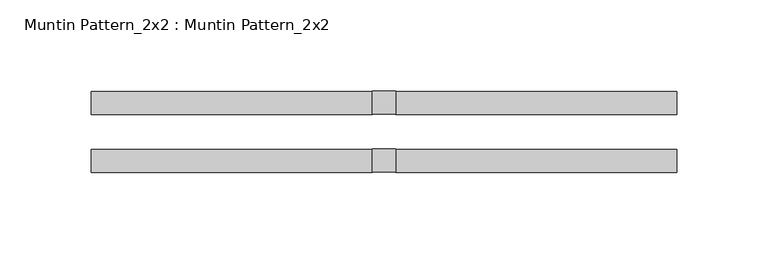
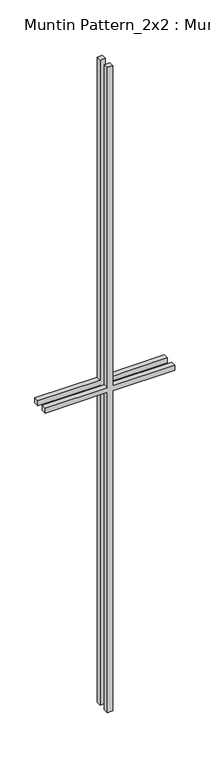
"""IFC4 building model written with IfcOpenShell, lengths in millimetres: proxy geometry, Muntin Pattern_2x2 : Muntin Pattern_2x2."""

from ifc_helpers import new_model, si_unit, frame, origin, place, context, project, spatial, polyline, outline, extrude, source, transform, mapped, element, save


def muntin_pattern_2x2_muntin_pattern_2x2_a158773a(model_context):
    return source(origin(), model_context, "Body", "SweptSolid", [
        extrude(outline(polyline([(850.9, -6.35), (850.9, -160.3375), (838.2, -160.3375), (838.2, -6.35), (0.0, -6.35), (0.0, 6.35), (838.2, 6.35), (838.2, 160.3375), (850.9, 160.3375), (850.9, 6.35), (1689.1, 6.35), (1689.1, -6.35), (850.9, -6.35)])), frame((0.0, 9.525, 0.0), z_axis=(0.0, 1.0, 0.0), x_axis=(0.0, 0.0, 1.0)), (0.0, 0.0, 1.0), 12.7),
        extrude(outline(polyline([(850.9, -6.35), (850.9, -160.3375), (838.2, -160.3375), (838.2, -6.35), (0.0, -6.35), (0.0, 6.35), (838.2, 6.35), (838.2, 160.3375), (850.9, 160.3375), (850.9, 6.35), (1689.1, 6.35), (1689.1, -6.35), (850.9, -6.35)])), frame((0.0, -22.225, 0.0), z_axis=(0.0, 1.0, 0.0), x_axis=(0.0, 0.0, 1.0)), (0.0, 0.0, 1.0), 12.7),
    ])


if __name__ == "__main__":
    model = new_model("IFC4")
    model_context = context("Model", 3, world=origin())
    ifc_project = project(units=[si_unit("LENGTHUNIT", "METRE", prefix="MILLI")], contexts=[model_context])
    site = spatial("IfcSite", under=ifc_project)
    building = spatial("IfcBuilding", under=site)
    placement = place(None, origin())
    muntin_pattern_2x2_muntin_pattern_2x2_shape = muntin_pattern_2x2_muntin_pattern_2x2_a158773a(model_context)
    element("IfcBuildingElementProxy", 1, Name="Muntin Pattern_2x2 : Muntin Pattern_2x2", ObjectType="Muntin Pattern_2x2 : Muntin Pattern_2x2", at=placement, inside=building, context=model_context, shape_type="MappedRepresentation", body=[
        mapped(muntin_pattern_2x2_muntin_pattern_2x2_shape, transform((0.0, 0.0, 0.0), x_axis=(1.0, 0.0, 0.0), y_axis=(0.0, 1.0, 0.0), z_axis=(0.0, 0.0, 1.0))),
    ])
    save(model, "model.ifc")

# Revit data of these elements
# Type "Muntin Pattern_2x2 : Muntin Pattern_2x2"
#   Width [instance default] = 4' - 0"
#   Thickness = 0' - 0 1/2"
#   Height [instance default] = 4' - 0"
#   Distance = 0' - 0 3/4"
#   Interior Material [instance default] = none
#   Exterior Material [instance default] = none
#   Default Elevation = 0
# Element 1 (IfcBuildingElementProxy, "Muntin Pattern_2x2 : Muntin Pattern_2x2")
#   Width = 1' - 0 5/8"
#   Height = 5' - 6 1/2"
#   Interior Material = Wood - Stained
#   Exterior Material = Clad - White
#   Materials on its faces: "Clad - White", "Wood - Stained"
# Materials
#   "Clad - White": class "Wood", colour RGB 242 242 238, transparency 0, Cost = 0
#   "Wood - Stained": class "Wood", colour RGB 224 178 126, transparency 0, Cost = 0
